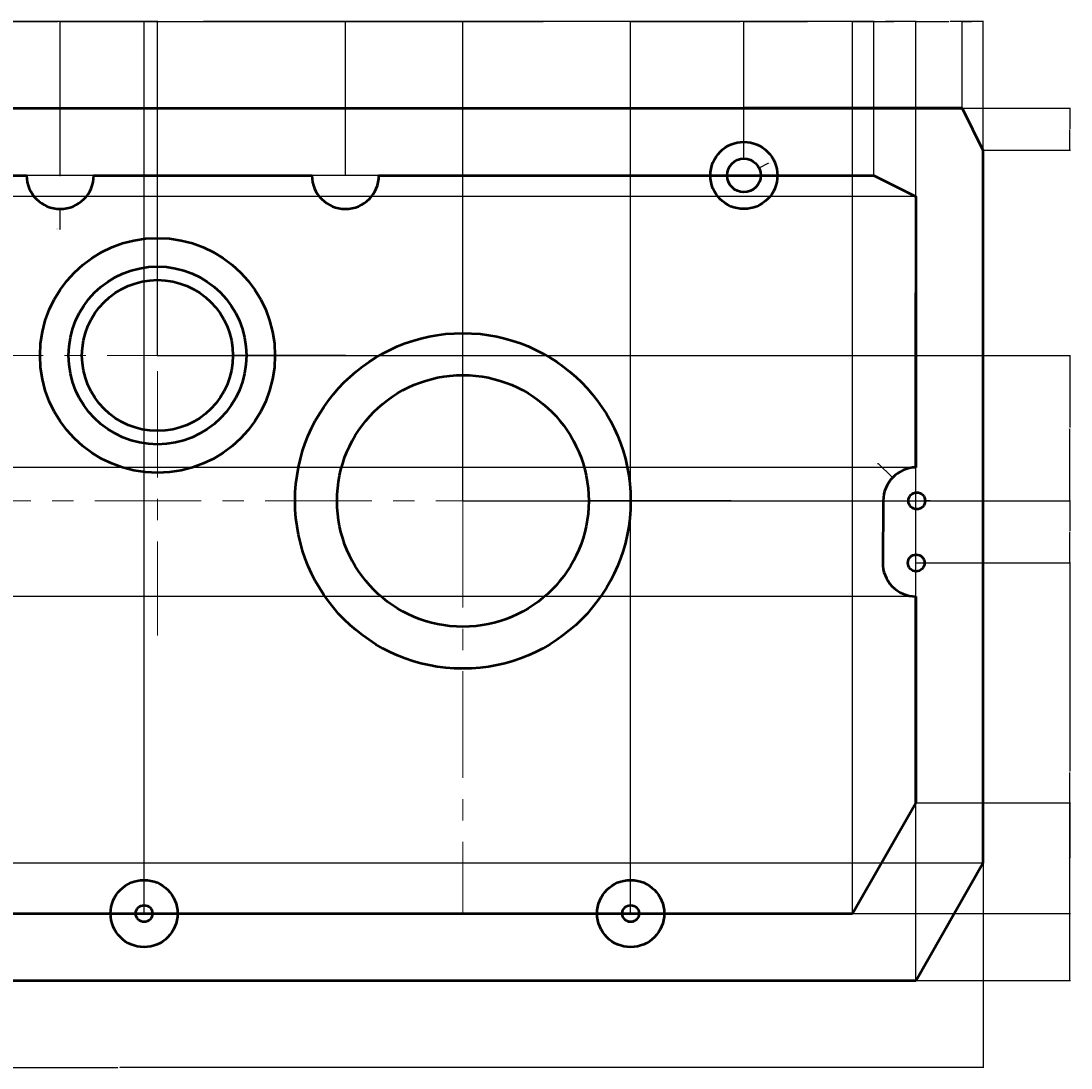
# Model space of a CAD drawing. Units: millimetres. Extents: x 2135 to 2702, y 2076 to 2388.
# Tile 2 of 2: x 2390 to 2702, y 2076 to 2388. Entities that reach past the tile are written whole.
import ezdxf

# ---------------------------------------------------------------- set-up
doc = ezdxf.new("R2010")
doc.units = ezdxf.units.MM
doc.linetypes.add('CENTER', pattern=[50.8, 31.75, -6.35, 6.35, -6.35])
for name, color, linetype, lineweight in [('M-CNTR', 4, 'CENTER', 18), ('M-DIMS', 2, 'Continuous', 18), ('M-OUTL', 7, 'Continuous', 50)]:
    doc.layers.add(name, color=color, linetype=linetype, lineweight=lineweight)
doc.styles.get("Standard").update_dxf_attribs({"font": 'arial.ttf'})
doc.dimstyles.get("Standard").update_dxf_attribs({"dimtxt": 0.18, "dimasz": 0.18, "dimexe": 0.18, "dimexo": 0.0625, "dimgap": 0.09, "dimtad": 0, "dimtih": 1, "dimtoh": 1, "dimdec": 4, "dimzin": 0, "dimdsep": 46, "dimtxsty": 'Standard', "dimcen": 0.09, "dimadec": 0, "dimazin": 0, "dimtfac": 1, "dimtdec": 4, "dimtofl": 0, "dimtmove": 0, "dimatfit": 3, "dimfxl": 1, "dimtolj": 1, "dimtzin": 0, "dimarcsym": 0})

# ---------------------------------------------------------------- blocks, each defined once
blk = doc.blocks.new('BOLT-HOLE-CBORE')
for radius in [10, 2.5]:
    blk.add_circle((10, 10), radius)
blk = doc.blocks.new('*D2')
at = {"layer": 'Defpoints', "color": 0, "transparency": 16777216}
for p in [(2676.22, 2136.75), (2161.22, 2101.69), (2676.22, 2075.84)]:
    blk.add_point(p, dxfattribs=at)
at = {"layer": 'M-DIMS', "color": 0, "lineweight": -2, "transparency": 16777216}
for p, q in [((2676.22, 2136.68), (2676.22, 2075.66)), ((2161.22, 2101.62), (2161.22, 2075.66)), ((2161.4, 2075.84), (2418.43, 2075.84)), ((2676.04, 2075.84), (2419.01, 2075.84))]:
    blk.add_line(p, q, dxfattribs=at)
at = {"layer": 'M-DIMS', "color": 0, "transparency": 16777216}
for points in [[(2161.4, 2075.87), (2161.4, 2075.81), (2161.22, 2075.84)], [(2676.04, 2075.87), (2676.04, 2075.81), (2676.22, 2075.84)]]:
    blk.add_solid(points, dxfattribs=at)
at = {"layer": 'M-DIMS', "color": 0, "transparency": 16777216, "insert": (2418.72, 2075.84), "char_height": 0.18, "attachment_point": 5}
blk.add_mtext('\\A1;515', dxfattribs=at)
blk = doc.blocks.new('*D6')
at = {"layer": 'Defpoints', "color": 0, "transparency": 16777216}
for p in [(2426.22, 2387.54), (2301.22, 2121.69), (2426.22, 2121.69)]:
    blk.add_point(p, dxfattribs=at)
at = {"layer": 'M-DIMS', "color": 0, "lineweight": -2, "transparency": 16777216}
for p, q in [((2301.22, 2121.75), (2301.22, 2387.72)), ((2301.4, 2387.54), (2363.44, 2387.54)), ((2426.04, 2387.54), (2364, 2387.54)), ((2426.22, 2121.75), (2426.22, 2387.72))]:
    blk.add_line(p, q, dxfattribs=at)
at = {"layer": 'M-DIMS', "color": 0, "transparency": 16777216}
for points in [[(2301.4, 2387.57), (2301.4, 2387.51), (2301.22, 2387.54)], [(2426.04, 2387.57), (2426.04, 2387.51), (2426.22, 2387.54)]]:
    blk.add_solid(points, dxfattribs=at)
at = {"layer": 'M-DIMS', "color": 0, "transparency": 16777216, "insert": (2363.72, 2387.54), "char_height": 0.18, "attachment_point": 5}
blk.add_mtext('\\A1;125', dxfattribs=at)
blk = doc.blocks.new('*D7')
at = {"layer": 'Defpoints', "color": 0, "transparency": 16777216}
for p in [(2571.22, 2387.54), (2426.22, 2121.69), (2571.22, 2121.69)]:
    blk.add_point(p, dxfattribs=at)
at = {"layer": 'M-DIMS', "color": 0, "lineweight": -2, "transparency": 16777216}
for p, q in [((2426.22, 2121.75), (2426.22, 2387.72)), ((2426.4, 2387.54), (2498.44, 2387.54)), ((2571.04, 2387.54), (2499, 2387.54)), ((2571.22, 2121.75), (2571.22, 2387.72))]:
    blk.add_line(p, q, dxfattribs=at)
at = {"layer": 'M-DIMS', "color": 0, "transparency": 16777216}
for points in [[(2426.4, 2387.57), (2426.4, 2387.51), (2426.22, 2387.54)], [(2571.04, 2387.57), (2571.04, 2387.51), (2571.22, 2387.54)]]:
    blk.add_solid(points, dxfattribs=at)
at = {"layer": 'M-DIMS', "color": 0, "transparency": 16777216, "insert": (2498.72, 2387.54), "char_height": 0.18, "attachment_point": 5}
blk.add_mtext('\\A1;145', dxfattribs=at)
blk = doc.blocks.new('*D8')
at = {"layer": 'Defpoints', "color": 0, "transparency": 16777216}
for p in [(2637.37, 2387.54), (2571.22, 2121.69), (2637.37, 2121.69)]:
    blk.add_point(p, dxfattribs=at)
at = {"layer": 'M-DIMS', "color": 0, "lineweight": -2, "transparency": 16777216}
for p, q in [((2571.22, 2121.75), (2571.22, 2387.72)), ((2571.4, 2387.54), (2603.9, 2387.54)), ((2637.19, 2387.54), (2604.69, 2387.54)), ((2637.37, 2121.75), (2637.37, 2387.72))]:
    blk.add_line(p, q, dxfattribs=at)
at = {"layer": 'M-DIMS', "color": 0, "transparency": 16777216}
for points in [[(2571.4, 2387.57), (2571.4, 2387.51), (2571.22, 2387.54)], [(2637.19, 2387.57), (2637.19, 2387.51), (2637.37, 2387.54)]]:
    blk.add_solid(points, dxfattribs=at)
at = {"layer": 'M-DIMS', "color": 0, "transparency": 16777216, "insert": (2604.29, 2387.54), "char_height": 0.18, "attachment_point": 5}
blk.add_mtext('\\A1;66.15', dxfattribs=at)
blk = doc.blocks.new('*D9')
at = {"layer": 'Defpoints', "color": 0, "transparency": 16777216}
for p in [(2656.22, 2387.54), (2656.22, 2154.73), (2637.37, 2121.69)]:
    blk.add_point(p, dxfattribs=at)
at = {"layer": 'M-DIMS', "color": 0, "lineweight": -2, "transparency": 16777216}
for p, q in [((2637.37, 2121.75), (2637.37, 2387.72)), ((2637.55, 2387.54), (2646.41, 2387.54)), ((2656.04, 2387.54), (2647.18, 2387.54)), ((2656.22, 2154.79), (2656.22, 2387.72))]:
    blk.add_line(p, q, dxfattribs=at)
at = {"layer": 'M-DIMS', "color": 0, "transparency": 16777216}
for points in [[(2637.55, 2387.57), (2637.55, 2387.51), (2637.37, 2387.54)], [(2656.04, 2387.57), (2656.04, 2387.51), (2656.22, 2387.54)]]:
    blk.add_solid(points, dxfattribs=at)
at = {"layer": 'M-DIMS', "color": 0, "transparency": 16777216, "insert": (2646.79, 2387.54), "char_height": 0.18, "attachment_point": 5}
blk.add_mtext('\\A1;18.85', dxfattribs=at)
blk = doc.blocks.new('*D10')
at = {"layer": 'Defpoints', "color": 0, "transparency": 16777216}
for p in [(2676.22, 2387.54), (2676.22, 2136.75), (2656.22, 2101.69)]:
    blk.add_point(p, dxfattribs=at)
at = {"layer": 'M-DIMS', "color": 0, "lineweight": -2, "transparency": 16777216}
for p, q in [((2656.22, 2101.75), (2656.22, 2387.72)), ((2656.4, 2387.54), (2666, 2387.54)), ((2676.04, 2387.54), (2666.44, 2387.54)), ((2676.22, 2136.81), (2676.22, 2387.72))]:
    blk.add_line(p, q, dxfattribs=at)
at = {"layer": 'M-DIMS', "color": 0, "transparency": 16777216}
for points in [[(2656.4, 2387.57), (2656.4, 2387.51), (2656.22, 2387.54)], [(2676.04, 2387.57), (2676.04, 2387.51), (2676.22, 2387.54)]]:
    blk.add_solid(points, dxfattribs=at)
at = {"layer": 'M-DIMS', "color": 0, "transparency": 16777216, "insert": (2666.22, 2387.54), "char_height": 0.18, "attachment_point": 5}
blk.add_mtext('\\A1;20', dxfattribs=at)
blk = doc.blocks.new('*D13')
at = {"layer": 'Defpoints', "color": 0, "transparency": 16777216}
for p in [(2401.22, 2387.54), (2371.22, 2341.69), (2401.22, 2341.69)]:
    blk.add_point(p, dxfattribs=at)
at = {"layer": 'M-DIMS', "color": 0, "lineweight": -2, "transparency": 16777216}
for p, q in [((2371.22, 2341.75), (2371.22, 2387.72)), ((2371.4, 2387.54), (2386, 2387.54)), ((2401.04, 2387.54), (2386.44, 2387.54)), ((2401.22, 2341.75), (2401.22, 2387.72))]:
    blk.add_line(p, q, dxfattribs=at)
at = {"layer": 'M-DIMS', "color": 0, "transparency": 16777216}
for points in [[(2371.4, 2387.57), (2371.4, 2387.51), (2371.22, 2387.54)], [(2401.04, 2387.57), (2401.04, 2387.51), (2401.22, 2387.54)]]:
    blk.add_solid(points, dxfattribs=at)
at = {"layer": 'M-DIMS', "color": 0, "transparency": 16777216, "insert": (2386.22, 2387.54), "char_height": 0.18, "attachment_point": 5}
blk.add_mtext('\\A1;30', dxfattribs=at)
blk = doc.blocks.new('*D14')
at = {"layer": 'Defpoints', "color": 0, "transparency": 16777216}
for p in [(2486.22, 2387.54), (2401.22, 2341.69), (2486.22, 2341.69)]:
    blk.add_point(p, dxfattribs=at)
at = {"layer": 'M-DIMS', "color": 0, "lineweight": -2, "transparency": 16777216}
for p, q in [((2401.22, 2341.75), (2401.22, 2387.72)), ((2401.4, 2387.54), (2443.5, 2387.54)), ((2486.04, 2387.54), (2443.94, 2387.54)), ((2486.22, 2341.75), (2486.22, 2387.72))]:
    blk.add_line(p, q, dxfattribs=at)
at = {"layer": 'M-DIMS', "color": 0, "transparency": 16777216}
for points in [[(2401.4, 2387.57), (2401.4, 2387.51), (2401.22, 2387.54)], [(2486.04, 2387.57), (2486.04, 2387.51), (2486.22, 2387.54)]]:
    blk.add_solid(points, dxfattribs=at)
at = {"layer": 'M-DIMS', "color": 0, "transparency": 16777216, "insert": (2443.72, 2387.54), "char_height": 0.18, "attachment_point": 5}
blk.add_mtext('\\A1;85', dxfattribs=at)
blk = doc.blocks.new('*D15')
at = {"layer": 'Defpoints', "color": 0, "transparency": 16777216}
for p in [(2604.97, 2387.54), (2604.97, 2346.69), (2486.22, 2341.69)]:
    blk.add_point(p, dxfattribs=at)
at = {"layer": 'M-DIMS', "color": 0, "lineweight": -2, "transparency": 16777216}
for p, q in [((2486.22, 2341.75), (2486.22, 2387.72)), ((2486.4, 2387.54), (2545.14, 2387.54)), ((2604.79, 2387.54), (2546.05, 2387.54)), ((2604.97, 2346.75), (2604.97, 2387.72))]:
    blk.add_line(p, q, dxfattribs=at)
at = {"layer": 'M-DIMS', "color": 0, "transparency": 16777216}
for points in [[(2486.4, 2387.57), (2486.4, 2387.51), (2486.22, 2387.54)], [(2604.79, 2387.57), (2604.79, 2387.51), (2604.97, 2387.54)]]:
    blk.add_solid(points, dxfattribs=at)
at = {"layer": 'M-DIMS', "color": 0, "transparency": 16777216, "insert": (2545.59, 2387.54), "char_height": 0.18, "attachment_point": 5}
blk.add_mtext('\\A1;118.75', dxfattribs=at)
blk = doc.blocks.new('*D16')
at = {"layer": 'Defpoints', "color": 0, "transparency": 16777216}
for p in [(2643.72, 2387.54), (2604.97, 2346.69), (2643.72, 2341.69)]:
    blk.add_point(p, dxfattribs=at)
at = {"layer": 'M-DIMS', "color": 0, "lineweight": -2, "transparency": 16777216}
for p, q in [((2604.97, 2346.75), (2604.97, 2387.72)), ((2605.15, 2387.54), (2623.95, 2387.54)), ((2643.54, 2387.54), (2624.74, 2387.54)), ((2643.72, 2341.75), (2643.72, 2387.72))]:
    blk.add_line(p, q, dxfattribs=at)
at = {"layer": 'M-DIMS', "color": 0, "transparency": 16777216}
for points in [[(2605.15, 2387.57), (2605.15, 2387.51), (2604.97, 2387.54)], [(2643.54, 2387.57), (2643.54, 2387.51), (2643.72, 2387.54)]]:
    blk.add_solid(points, dxfattribs=at)
at = {"layer": 'M-DIMS', "color": 0, "transparency": 16777216, "insert": (2624.34, 2387.54), "char_height": 0.18, "attachment_point": 5}
blk.add_mtext('\\A1;38.75', dxfattribs=at)
blk = doc.blocks.new('*D17')
at = {"layer": 'Defpoints', "color": 0, "transparency": 16777216}
for p in [(2656.22, 2387.54), (2643.72, 2341.69), (2656.22, 2335.44)]:
    blk.add_point(p, dxfattribs=at)
at = {"layer": 'M-DIMS', "color": 0, "lineweight": -2, "transparency": 16777216}
for p, q in [((2643.72, 2341.75), (2643.72, 2387.72)), ((2643.9, 2387.54), (2649.65, 2387.54)), ((2656.04, 2387.54), (2650.28, 2387.54)), ((2656.22, 2335.5), (2656.22, 2387.72))]:
    blk.add_line(p, q, dxfattribs=at)
at = {"layer": 'M-DIMS', "color": 0, "transparency": 16777216}
for points in [[(2643.9, 2387.57), (2643.9, 2387.51), (2643.72, 2387.54)], [(2656.04, 2387.57), (2656.04, 2387.51), (2656.22, 2387.54)]]:
    blk.add_solid(points, dxfattribs=at)
at = {"layer": 'M-DIMS', "color": 0, "transparency": 16777216, "insert": (2649.97, 2387.54), "char_height": 0.18, "attachment_point": 5}
blk.add_mtext('\\A1;12.5', dxfattribs=at)
blk = doc.blocks.new('*D18')
at = {"layer": 'Defpoints', "color": 0, "transparency": 16777216}
for p in [(2676.22, 2387.54), (2669.97, 2361.69), (2676.22, 2349.19)]:
    blk.add_point(p, dxfattribs=at)
at = {"layer": 'M-DIMS', "color": 0, "lineweight": -2, "transparency": 16777216}
for p, q in [((2669.97, 2361.75), (2669.97, 2387.72)), ((2670.15, 2387.54), (2672.77, 2387.54)), ((2676.04, 2387.54), (2673.42, 2387.54)), ((2676.22, 2349.25), (2676.22, 2387.72))]:
    blk.add_line(p, q, dxfattribs=at)
at = {"layer": 'M-DIMS', "color": 0, "transparency": 16777216}
for points in [[(2670.15, 2387.57), (2670.15, 2387.51), (2669.97, 2387.54)], [(2676.04, 2387.57), (2676.04, 2387.51), (2676.22, 2387.54)]]:
    blk.add_solid(points, dxfattribs=at)
at = {"layer": 'M-DIMS', "color": 0, "transparency": 16777216, "insert": (2673.09, 2387.54), "char_height": 0.18, "attachment_point": 5}
blk.add_mtext('\\A1;6.25', dxfattribs=at)
blk = doc.blocks.new('*D19')
at = {"layer": 'Defpoints', "color": 0, "transparency": 16777216}
for p in [(2430.22, 2387.54), (2371.22, 2306.69), (2430.22, 2288.03)]:
    blk.add_point(p, dxfattribs=at)
at = {"layer": 'M-DIMS', "color": 0, "lineweight": -2, "transparency": 16777216}
for p, q in [((2371.22, 2306.75), (2371.22, 2387.72)), ((2371.4, 2387.54), (2400.5, 2387.54)), ((2430.04, 2387.54), (2400.94, 2387.54)), ((2430.22, 2288.1), (2430.22, 2387.72))]:
    blk.add_line(p, q, dxfattribs=at)
at = {"layer": 'M-DIMS', "color": 0, "transparency": 16777216}
for points in [[(2371.4, 2387.57), (2371.4, 2387.51), (2371.22, 2387.54)], [(2430.04, 2387.57), (2430.04, 2387.51), (2430.22, 2387.54)]]:
    blk.add_solid(points, dxfattribs=at)
at = {"layer": 'M-DIMS', "color": 0, "transparency": 16777216, "insert": (2400.72, 2387.54), "char_height": 0.18, "attachment_point": 5}
blk.add_mtext('\\A1;59', dxfattribs=at)
blk = doc.blocks.new('*D20')
at = {"layer": 'Defpoints', "color": 0, "transparency": 16777216}
for p in [(2521.22, 2387.54), (2430.22, 2288.03), (2521.22, 2244.69)]:
    blk.add_point(p, dxfattribs=at)
at = {"layer": 'M-DIMS', "color": 0, "lineweight": -2, "transparency": 16777216}
for p, q in [((2430.22, 2288.1), (2430.22, 2387.72)), ((2430.4, 2387.54), (2475.52, 2387.54)), ((2521.04, 2387.54), (2475.92, 2387.54)), ((2521.22, 2244.75), (2521.22, 2387.72))]:
    blk.add_line(p, q, dxfattribs=at)
at = {"layer": 'M-DIMS', "color": 0, "transparency": 16777216}
for points in [[(2430.4, 2387.57), (2430.4, 2387.51), (2430.22, 2387.54)], [(2521.04, 2387.57), (2521.04, 2387.51), (2521.22, 2387.54)]]:
    blk.add_solid(points, dxfattribs=at)
at = {"layer": 'M-DIMS', "color": 0, "transparency": 16777216, "insert": (2475.72, 2387.54), "char_height": 0.18, "attachment_point": 5}
blk.add_mtext('\\A1;91', dxfattribs=at)
blk = doc.blocks.new('*D22')
at = {"layer": 'Defpoints', "color": 0, "transparency": 16777216}
for p in [(2637.37, 2121.69), (2135.37, 2101.69), (2656.22, 2101.69)]:
    blk.add_point(p, dxfattribs=at)
at = {"layer": 'M-DIMS', "color": 0, "lineweight": -2, "transparency": 16777216}
for p, q in [((2637.3, 2121.69), (2135.19, 2121.69)), ((2135.37, 2121.51), (2135.37, 2111.87)), ((2135.37, 2101.87), (2135.37, 2111.5)), ((2656.15, 2101.69), (2135.19, 2101.69))]:
    blk.add_line(p, q, dxfattribs=at)
at = {"layer": 'M-DIMS', "color": 0, "transparency": 16777216}
for points in [[(2135.34, 2121.51), (2135.4, 2121.51), (2135.37, 2121.69)], [(2135.34, 2101.87), (2135.4, 2101.87), (2135.37, 2101.69)]]:
    blk.add_solid(points, dxfattribs=at)
at = {"layer": 'M-DIMS', "color": 0, "transparency": 16777216, "insert": (2135.37, 2111.69), "char_height": 0.18, "attachment_point": 5}
blk.add_mtext('\\A1;20', dxfattribs=at)
blk = doc.blocks.new('*D27')
at = {"layer": 'Defpoints', "color": 0, "transparency": 16777216}
for p in [(2656.33, 2226.19), (2702.07, 2226.19), (2656.22, 2101.69)]:
    blk.add_point(p, dxfattribs=at)
at = {"layer": 'M-DIMS', "color": 0, "lineweight": -2, "transparency": 16777216}
for p, q in [((2656.39, 2226.19), (2702.25, 2226.19)), ((2702.07, 2226.01), (2702.07, 2164.12)), ((2702.07, 2101.87), (2702.07, 2163.75)), ((2656.28, 2101.69), (2702.25, 2101.69))]:
    blk.add_line(p, q, dxfattribs=at)
at = {"layer": 'M-DIMS', "color": 0, "transparency": 16777216}
for points in [[(2702.04, 2226.01), (2702.1, 2226.01), (2702.07, 2226.19)], [(2702.04, 2101.87), (2702.1, 2101.87), (2702.07, 2101.69)]]:
    blk.add_solid(points, dxfattribs=at)
at = {"layer": 'M-DIMS', "color": 0, "transparency": 16777216, "insert": (2702.07, 2163.94), "char_height": 0.18, "attachment_point": 5}
blk.add_mtext('\\A1;124.5', dxfattribs=at)
blk = doc.blocks.new('*D28')
at = {"layer": 'Defpoints', "color": 0, "transparency": 16777216}
for p in [(2521.22, 2244.69), (2702.07, 2244.69), (2656.33, 2226.19)]:
    blk.add_point(p, dxfattribs=at)
at = {"layer": 'M-DIMS', "color": 0, "lineweight": -2, "transparency": 16777216}
for p, q in [((2521.28, 2244.69), (2702.25, 2244.69)), ((2702.07, 2244.51), (2702.07, 2235.62)), ((2702.07, 2226.37), (2702.07, 2235.25)), ((2656.39, 2226.19), (2702.25, 2226.19))]:
    blk.add_line(p, q, dxfattribs=at)
at = {"layer": 'M-DIMS', "color": 0, "transparency": 16777216}
for points in [[(2702.04, 2244.51), (2702.1, 2244.51), (2702.07, 2244.69)], [(2702.04, 2226.37), (2702.1, 2226.37), (2702.07, 2226.19)]]:
    blk.add_solid(points, dxfattribs=at)
at = {"layer": 'M-DIMS', "color": 0, "transparency": 16777216, "insert": (2702.07, 2235.44), "char_height": 0.18, "attachment_point": 5}
blk.add_mtext('\\A1;18.5', dxfattribs=at)
blk = doc.blocks.new('*D29')
at = {"layer": 'Defpoints', "color": 0, "transparency": 16777216}
for p in [(2430.22, 2288.03), (2702.07, 2288.03), (2521.22, 2244.69)]:
    blk.add_point(p, dxfattribs=at)
at = {"layer": 'M-DIMS', "color": 0, "lineweight": -2, "transparency": 16777216}
for p, q in [((2430.28, 2288.03), (2702.25, 2288.03)), ((2702.07, 2287.85), (2702.07, 2266.54)), ((2702.07, 2244.87), (2702.07, 2266.18)), ((2521.28, 2244.69), (2702.25, 2244.69))]:
    blk.add_line(p, q, dxfattribs=at)
at = {"layer": 'M-DIMS', "color": 0, "transparency": 16777216}
for points in [[(2702.04, 2287.85), (2702.1, 2287.85), (2702.07, 2288.03)], [(2702.04, 2244.87), (2702.1, 2244.87), (2702.07, 2244.69)]]:
    blk.add_solid(points, dxfattribs=at)
at = {"layer": 'M-DIMS', "color": 0, "transparency": 16777216, "insert": (2702.07, 2266.36), "char_height": 0.18, "attachment_point": 5}
blk.add_mtext('\\A1;43.35', dxfattribs=at)
blk = doc.blocks.new('*D30')
at = {"layer": 'Defpoints', "color": 0, "transparency": 16777216}
for p in [(2135.37, 2254.68), (2656.22, 2254.68), (2656.22, 2216.19)]:
    blk.add_point(p, dxfattribs=at)
at = {"layer": 'M-DIMS', "color": 0, "lineweight": -2, "transparency": 16777216}
for p, q in [((2656.15, 2254.68), (2135.19, 2254.68)), ((2135.37, 2254.5), (2135.37, 2235.62)), ((2135.37, 2216.37), (2135.37, 2235.25)), ((2656.15, 2216.19), (2135.19, 2216.19))]:
    blk.add_line(p, q, dxfattribs=at)
at = {"layer": 'M-DIMS', "color": 0, "transparency": 16777216}
for points in [[(2135.34, 2254.5), (2135.4, 2254.5), (2135.37, 2254.68)], [(2135.34, 2216.37), (2135.4, 2216.37), (2135.37, 2216.19)]]:
    blk.add_solid(points, dxfattribs=at)
at = {"layer": 'M-DIMS', "color": 0, "transparency": 16777216, "insert": (2135.37, 2235.43), "char_height": 0.18, "attachment_point": 5}
blk.add_mtext('\\A1;38.495', dxfattribs=at)
blk = doc.blocks.new('*D31')
at = {"layer": 'Defpoints', "color": 0, "transparency": 16777216}
for p in [(2135.37, 2136.75), (2676.22, 2136.75), (2656.22, 2101.69)]:
    blk.add_point(p, dxfattribs=at)
at = {"layer": 'M-DIMS', "color": 0, "lineweight": -2, "transparency": 16777216}
for p, q in [((2676.15, 2136.75), (2135.19, 2136.75)), ((2135.37, 2136.57), (2135.37, 2119.4)), ((2135.37, 2101.87), (2135.37, 2119.03)), ((2656.15, 2101.69), (2135.19, 2101.69))]:
    blk.add_line(p, q, dxfattribs=at)
at = {"layer": 'M-DIMS', "color": 0, "transparency": 16777216}
for points in [[(2135.34, 2136.57), (2135.4, 2136.57), (2135.37, 2136.75)], [(2135.34, 2101.87), (2135.4, 2101.87), (2135.37, 2101.69)]]:
    blk.add_solid(points, dxfattribs=at)
at = {"layer": 'M-DIMS', "color": 0, "transparency": 16777216, "insert": (2135.37, 2119.22), "char_height": 0.18, "attachment_point": 5}
blk.add_mtext('\\A1;35.06', dxfattribs=at)
blk = doc.blocks.new('*D32')
at = {"layer": 'Defpoints', "color": 0, "transparency": 16777216}
for p in [(2656.22, 2154.73), (2702.07, 2154.73), (2637.37, 2121.69)]:
    blk.add_point(p, dxfattribs=at)
at = {"layer": 'M-DIMS', "color": 0, "lineweight": -2, "transparency": 16777216}
for p, q in [((2656.28, 2154.73), (2702.25, 2154.73)), ((2702.07, 2154.55), (2702.07, 2138.39)), ((2702.07, 2121.87), (2702.07, 2138.03)), ((2637.43, 2121.69), (2702.25, 2121.69))]:
    blk.add_line(p, q, dxfattribs=at)
at = {"layer": 'M-DIMS', "color": 0, "transparency": 16777216}
for points in [[(2702.04, 2154.55), (2702.1, 2154.55), (2702.07, 2154.73)], [(2702.04, 2121.87), (2702.1, 2121.87), (2702.07, 2121.69)]]:
    blk.add_solid(points, dxfattribs=at)
at = {"layer": 'M-DIMS', "color": 0, "transparency": 16777216, "insert": (2702.07, 2138.21), "char_height": 0.18, "attachment_point": 5}
blk.add_mtext('\\A1;33.045', dxfattribs=at)
blk = doc.blocks.new('*D33')
at = {"layer": 'Defpoints', "color": 0, "transparency": 16777216}
for p in [(2669.97, 2361.69), (2676.22, 2349.19), (2702.07, 2349.19)]:
    blk.add_point(p, dxfattribs=at)
at = {"layer": 'M-DIMS', "color": 0, "lineweight": -2, "transparency": 16777216}
for p, q in [((2670.03, 2361.69), (2702.25, 2361.69)), ((2702.07, 2361.51), (2702.07, 2355.62)), ((2702.07, 2349.37), (2702.07, 2355.25)), ((2676.28, 2349.19), (2702.25, 2349.19))]:
    blk.add_line(p, q, dxfattribs=at)
at = {"layer": 'M-DIMS', "color": 0, "transparency": 16777216}
for points in [[(2702.04, 2361.51), (2702.1, 2361.51), (2702.07, 2361.69)], [(2702.04, 2349.37), (2702.1, 2349.37), (2702.07, 2349.19)]]:
    blk.add_solid(points, dxfattribs=at)
at = {"layer": 'M-DIMS', "color": 0, "transparency": 16777216, "insert": (2702.07, 2355.44), "char_height": 0.18, "attachment_point": 5}
blk.add_mtext('\\A1;12.5', dxfattribs=at)
blk = doc.blocks.new('*D34')
at = {"layer": 'Defpoints', "color": 0, "transparency": 16777216}
for p in [(2643.72, 2341.69), (2135.37, 2335.44), (2656.22, 2335.44)]:
    blk.add_point(p, dxfattribs=at)
at = {"layer": 'M-DIMS', "color": 0, "lineweight": -2, "transparency": 16777216}
for p, q in [((2643.65, 2341.69), (2135.19, 2341.69)), ((2135.37, 2341.51), (2135.37, 2338.74)), ((2135.37, 2335.62), (2135.37, 2338.38)), ((2656.15, 2335.44), (2135.19, 2335.44))]:
    blk.add_line(p, q, dxfattribs=at)
at = {"layer": 'M-DIMS', "color": 0, "transparency": 16777216}
for points in [[(2135.34, 2341.51), (2135.4, 2341.51), (2135.37, 2341.69)], [(2135.34, 2335.62), (2135.4, 2335.62), (2135.37, 2335.44)]]:
    blk.add_solid(points, dxfattribs=at)
at = {"layer": 'M-DIMS', "color": 0, "transparency": 16777216, "insert": (2135.37, 2338.56), "char_height": 0.18, "attachment_point": 5}
blk.add_mtext('\\A1;6.25', dxfattribs=at)
blk = doc.blocks.new('*D35')
at = {"layer": 'Defpoints', "color": 0, "transparency": 16777216}
for p in [(2471.22, 2244.67), (2571.22, 2244.7)]:
    blk.add_point(p, dxfattribs=at)
at = {"layer": 'M-DIMS', "color": 0, "lineweight": -2, "transparency": 16777216}
for p, q in [((2521.13, 2244.69), (2521.31, 2244.69)), ((2521.22, 2244.6), (2521.22, 2244.78)), ((2601.22, 2244.71), (2571.4, 2244.7))]:
    blk.add_line(p, q, dxfattribs=at)
at = {"layer": 'M-DIMS', "color": 0, "transparency": 16777216}
blk.add_solid([(2571.4, 2244.73), (2571.4, 2244.67), (2571.22, 2244.7)], dxfattribs=at)
at = {"layer": 'M-DIMS', "color": 0, "transparency": 16777216, "insert": (2601.6, 2244.71), "char_height": 0.18, "attachment_point": 5}
blk.add_mtext('\\A1;∅100', dxfattribs=at)
blk = doc.blocks.new('*D36')
at = {"layer": 'Defpoints', "color": 0, "transparency": 16777216}
for p in [(2483.72, 2244.67), (2558.72, 2244.7)]:
    blk.add_point(p, dxfattribs=at)
at = {"layer": 'M-DIMS', "color": 0, "lineweight": -2, "transparency": 16777216}
for p, q in [((2521.13, 2244.69), (2521.31, 2244.69)), ((2521.22, 2244.6), (2521.22, 2244.78)), ((2581.22, 2244.71), (2558.9, 2244.7))]:
    blk.add_line(p, q, dxfattribs=at)
at = {"layer": 'M-DIMS', "color": 0, "transparency": 16777216}
blk.add_solid([(2558.9, 2244.73), (2558.9, 2244.67), (2558.72, 2244.7)], dxfattribs=at)
at = {"layer": 'M-DIMS', "color": 0, "transparency": 16777216, "insert": (2581.53, 2244.71), "char_height": 0.18, "attachment_point": 5}
blk.add_mtext('\\A1;∅75', dxfattribs=at)
blk = doc.blocks.new('*D37')
at = {"layer": 'Defpoints', "color": 0, "transparency": 16777216}
for p in [(2395.22, 2288.07), (2465.22, 2288)]:
    blk.add_point(p, dxfattribs=at)
at = {"layer": 'M-DIMS', "color": 0, "lineweight": -2, "transparency": 16777216}
for p, q in [((2430.13, 2288.03), (2430.31, 2288.03)), ((2430.22, 2287.94), (2430.22, 2288.12)), ((2486.22, 2287.98), (2465.4, 2288))]:
    blk.add_line(p, q, dxfattribs=at)
at = {"layer": 'M-DIMS', "color": 0, "transparency": 16777216}
blk.add_solid([(2465.4, 2288.03), (2465.4, 2287.97), (2465.22, 2288)], dxfattribs=at)
at = {"layer": 'M-DIMS', "color": 0, "transparency": 16777216, "insert": (2486.53, 2287.98), "char_height": 0.18, "attachment_point": 5}
blk.add_mtext('\\A1;∅70', dxfattribs=at)
blk = doc.blocks.new('*D38')
at = {"layer": 'Defpoints', "color": 0, "transparency": 16777216}
for p in [(2403.72, 2288.07), (2456.72, 2288)]:
    blk.add_point(p, dxfattribs=at)
at = {"layer": 'M-DIMS', "color": 0, "lineweight": -2, "transparency": 16777216}
for p, q in [((2430.13, 2288.03), (2430.31, 2288.03)), ((2430.22, 2287.94), (2430.22, 2288.12)), ((2472.62, 2287.98), (2456.9, 2288))]:
    blk.add_line(p, q, dxfattribs=at)
at = {"layer": 'M-DIMS', "color": 0, "transparency": 16777216}
blk.add_solid([(2456.9, 2288.03), (2456.9, 2287.97), (2456.72, 2288)], dxfattribs=at)
at = {"layer": 'M-DIMS', "color": 0, "transparency": 16777216, "insert": (2472.93, 2287.98), "char_height": 0.18, "attachment_point": 5}
blk.add_mtext('\\A1;∅53', dxfattribs=at)
blk = doc.blocks.new('*D39')
at = {"layer": 'Defpoints', "color": 0, "transparency": 16777216}
for p in [(2407.72, 2288.07), (2452.72, 2288)]:
    blk.add_point(p, dxfattribs=at)
at = {"layer": 'M-DIMS', "color": 0, "lineweight": -2, "transparency": 16777216}
for p, q in [((2430.13, 2288.03), (2430.31, 2288.03)), ((2430.22, 2287.94), (2430.22, 2288.12)), ((2466.22, 2287.98), (2452.9, 2288))]:
    blk.add_line(p, q, dxfattribs=at)
at = {"layer": 'M-DIMS', "color": 0, "transparency": 16777216}
blk.add_solid([(2452.9, 2288.03), (2452.9, 2287.97), (2452.72, 2288)], dxfattribs=at)
at = {"layer": 'M-DIMS', "color": 0, "transparency": 16777216, "insert": (2466.53, 2287.98), "char_height": 0.18, "attachment_point": 5}
blk.add_mtext('\\A1;∅45', dxfattribs=at)
blk = doc.blocks.new('*D40')
at = {"layer": 'Defpoints', "color": 0, "transparency": 16777216}
for p in [(2416.22, 2121.67), (2436.22, 2121.7)]:
    blk.add_point(p, dxfattribs=at)
at = {"layer": 'M-DIMS', "color": 0, "lineweight": -2, "transparency": 16777216}
for p, q in [((2426.13, 2121.69), (2426.31, 2121.69)), ((2426.22, 2121.6), (2426.22, 2121.78)), ((2442.22, 2121.71), (2436.4, 2121.7))]:
    blk.add_line(p, q, dxfattribs=at)
at = {"layer": 'M-DIMS', "color": 0, "transparency": 16777216}
blk.add_solid([(2436.4, 2121.73), (2436.4, 2121.67), (2436.22, 2121.7)], dxfattribs=at)
at = {"layer": 'M-DIMS', "color": 0, "transparency": 16777216, "insert": (2442.73, 2121.71), "char_height": 0.18, "attachment_point": 5}
blk.add_mtext('\\A1;4X ∅20', dxfattribs=at)
blk = doc.blocks.new('*D42')
at = {"layer": 'Defpoints', "color": 0, "transparency": 16777216}
for p in [(2609.44, 2343.92), (2600.49, 2339.45)]:
    blk.add_point(p, dxfattribs=at)
at = {"layer": 'M-DIMS', "color": 0, "lineweight": -2, "transparency": 16777216}
for p, q in [((2612.12, 2345.26), (2609.6, 2344)), ((2612.3, 2345.26), (2612.12, 2345.26)), ((2604.88, 2341.69), (2605.06, 2341.69)), ((2604.97, 2341.6), (2604.97, 2341.78))]:
    blk.add_line(p, q, dxfattribs=at)
at = {"layer": 'M-DIMS', "color": 0, "transparency": 16777216}
blk.add_solid([(2609.59, 2344.03), (2609.61, 2343.97), (2609.44, 2343.92)], dxfattribs=at)
at = {"layer": 'M-DIMS', "color": 0, "transparency": 16777216, "insert": (2612.62, 2345.26), "char_height": 0.18, "attachment_point": 5}
blk.add_mtext('\\A1;∅10', dxfattribs=at)
blk = doc.blocks.new('*D45')
at = {"layer": 'Defpoints', "color": 0, "transparency": 16777216}
for p in [(2653.98, 2244.67), (2658.98, 2244.7)]:
    blk.add_point(p, dxfattribs=at)
at = {"layer": 'M-DIMS', "color": 0, "lineweight": -2, "transparency": 16777216}
for p, q in [((2656.39, 2244.69), (2656.57, 2244.69)), ((2656.48, 2244.6), (2656.48, 2244.78)), ((2660.48, 2244.71), (2659.16, 2244.7))]:
    blk.add_line(p, q, dxfattribs=at)
at = {"layer": 'M-DIMS', "color": 0, "transparency": 16777216}
blk.add_solid([(2659.16, 2244.73), (2659.16, 2244.67), (2658.98, 2244.7)], dxfattribs=at)
at = {"layer": 'M-DIMS', "color": 0, "transparency": 16777216, "insert": (2660.91, 2244.71), "char_height": 0.18, "attachment_point": 5}
blk.add_mtext('\\A1;2X ∅5', dxfattribs=at)
blk = doc.blocks.new('*D46')
at = {"layer": 'Defpoints', "color": 0, "transparency": 16777216}
for p in [(2401.22, 2341.69), (2401.19, 2331.69)]:
    blk.add_point(p, dxfattribs=at)
at = {"layer": 'M-DIMS', "color": 0, "lineweight": -2, "transparency": 16777216}
for p, q in [((2401.13, 2341.69), (2401.31, 2341.69)), ((2401.22, 2341.6), (2401.22, 2341.78)), ((2401.18, 2325.69), (2401.19, 2331.51)), ((2401, 2325.69), (2401.18, 2325.69))]:
    blk.add_line(p, q, dxfattribs=at)
at = {"layer": 'M-DIMS', "color": 0, "transparency": 16777216}
blk.add_solid([(2401.16, 2331.51), (2401.22, 2331.51), (2401.19, 2331.69)], dxfattribs=at)
at = {"layer": 'M-DIMS', "color": 0, "transparency": 16777216, "insert": (2400.5, 2325.69), "char_height": 0.18, "attachment_point": 5}
blk.add_mtext('\\A1;3X R10', dxfattribs=at)
blk = doc.blocks.new('*D47')
at = {"layer": 'Defpoints', "color": 0, "transparency": 16777216}
for p in [(2649.28, 2251.63), (2656.48, 2244.69)]:
    blk.add_point(p, dxfattribs=at)
at = {"layer": 'M-DIMS', "color": 0, "lineweight": -2, "transparency": 16777216}
for p, q in [((2644.78, 2255.79), (2644.96, 2255.79)), ((2644.96, 2255.79), (2649.15, 2251.75)), ((2656.39, 2244.69), (2656.57, 2244.69)), ((2656.48, 2244.6), (2656.48, 2244.78))]:
    blk.add_line(p, q, dxfattribs=at)
at = {"layer": 'M-DIMS', "color": 0, "transparency": 16777216}
blk.add_solid([(2649.17, 2251.77), (2649.13, 2251.73), (2649.28, 2251.63)], dxfattribs=at)
at = {"layer": 'M-DIMS', "color": 0, "transparency": 16777216, "insert": (2644.28, 2255.79), "char_height": 0.18, "attachment_point": 5}
blk.add_mtext('\\A1;2X R10', dxfattribs=at)

msp = doc.modelspace()

# ---------------------------------------------------------------- linework, layer by layer
at = {"layer": 'M-CNTR'}
for p, q in [((2430.2172, 2334.1854), (2430.2172, 2204.5212)), ((2161.2172, 2288.0325), (2416.86, 2288.0325)), ((2416.86, 2288.0325), (2456.1851, 2288.0325)), ((2646.4762, 2244.6854), (2292.5799, 2244.6854))]:
    msp.add_line(p, q, dxfattribs=at)
msp.add_lwpolyline([(2521.2172, 2244.6854), (2521.2172, 2121.6854)], dxfattribs=at)
at = {"layer": 'M-OUTL'}
for p, q in [((2669.9672, 2361.6854), (2604.9672, 2361.6854)), ((2676.2172, 2341.6854), (2676.2172, 2244.6854)), ((2646.4762, 2244.6854), (2646.3257, 2226.186)), ((2637.3663, 2121.6854), (2656.2172, 2154.7307)), ((2656.2172, 2101.6854), (2676.2172, 2136.745))]:
    msp.add_line(p, q, dxfattribs=at)
for points in [[(2656.2172, 2101.6854), (2161.2172, 2101.6854), (2161.2172, 2121.6854), (2161.2172, 2324.3525), (2161.2172, 2326.6854), (2181.2172, 2326.6854), (2351.2172, 2326.6854), (2351.2172, 2341.6854), (2351.2172, 2361.6854), (2371.2172, 2361.6854), (2669.9672, 2361.6854), (2676.2172, 2349.1854), (2676.2172, 2341.6854), (2676.2172, 2136.745)], [(2656.2172, 2254.6821), (2656.2172, 2306.6854)], [(2656.2172, 2154.7307), (2656.2172, 2216.1866)], [(2656.2172, 2216.1866), (2656.2172, 2154.7307)]]:
    msp.add_lwpolyline(points, dxfattribs=at)
for points in [[(2371.2172, 2306.6854), (2371.2172, 2341.6854), (2391.2172, 2341.6854, 1), (2411.2172, 2341.6854), (2476.2172, 2341.6854, 1), (2496.2172, 2341.6854), (2643.7172, 2341.6854), (2656.2172, 2335.4354), (2656.2172, 2254.6821)], [(2181.2172, 2226.6854), (2181.2172, 2131.6854, -0.41421356), (2191.2172, 2121.6854), (2637.3663, 2121.6854)]]:
    msp.add_lwpolyline(points, format="xyb", dxfattribs=at)
for centre, radius in [((2604.9672, 2341.6854), 10), ((2604.9672, 2341.6854), 5), ((2430.2172, 2288.0325), 35), ((2430.2172, 2288.0325), 26.5), ((2430.2172, 2288.0325), 22.5), ((2521.2172, 2244.6854), 50), ((2521.2172, 2244.6854), 37.5), ((2656.4762, 2244.6854), 2.5), ((2656.3257, 2226.186), 2.5)]:
    msp.add_circle(centre, radius, dxfattribs=at)
for centre, start, end in [((2656.4762, 2244.6854), 91.483946, 180), ((2656.3257, 2226.186), 179.067727, 269.37855)]:
    msp.add_arc(centre, 10, start, end, dxfattribs=at)

# ---------------------------------------------------------------- block references
for p in [(2416.217, 2111.685), (2561.217, 2111.685)]:
    msp.add_blockref('BOLT-HOLE-CBORE', p, dxfattribs=at)

# ---------------------------------------------------------------- dimensions: what is measured, and where the dimension line sits
at = {"layer": 'M-DIMS'}
for base, p1, p2, override, picture, middle in [((2426.2172, 2387.5354), (2301.2172, 2121.6854), (2426.2172, 2121.6854), {"dimdec": 0, "dimlfac": 1, "dimrnd": 0, "dimzin": 0, "dimdsep": 46, "dimlunit": 2}, '*D6', (2363.7172, 2387.5354)), ((2401.2172, 2387.5354), (2371.2172, 2341.6854), (2401.2172, 2341.6854), {"dimdec": 0, "dimlfac": 1, "dimrnd": 0, "dimzin": 0, "dimdsep": 46, "dimlunit": 2}, '*D13', (2386.2172, 2387.5354)), ((2430.2172, 2387.5354), (2371.2172, 2306.6854), (2430.2172, 2288.0325), {"dimdec": 0, "dimlfac": 1, "dimrnd": 0, "dimzin": 0, "dimdsep": 46, "dimlunit": 2}, '*D19', (2400.7172, 2387.5354)), ((2486.2172, 2387.5354), (2401.2172, 2341.6854), (2486.2172, 2341.6854), {"dimdec": 0, "dimlfac": 1, "dimrnd": 0, "dimzin": 0, "dimdsep": 46, "dimlunit": 2}, '*D14', (2443.7172, 2387.5354)), ((2571.2172, 2387.5354), (2426.2172, 2121.6854), (2571.2172, 2121.6854), {"dimdec": 0, "dimlfac": 1, "dimrnd": 0, "dimzin": 0, "dimdsep": 46, "dimlunit": 2}, '*D7', (2498.7172, 2387.5354)), ((2521.2172, 2387.5354), (2430.2172, 2288.0325), (2521.2172, 2244.6854), {"dimdec": 0, "dimlfac": 1, "dimrnd": 0, "dimzin": 0, "dimdsep": 46, "dimlunit": 2}, '*D20', (2475.7172, 2387.5354)), ((2604.9672, 2387.5354), (2486.2172, 2341.6854), (2604.9672, 2346.6854), {"dimdec": 2, "dimlfac": 1, "dimrnd": 0, "dimzin": 0, "dimdsep": 46, "dimlunit": 2}, '*D15', (2545.5922, 2387.5354)), ((2637.3663, 2387.5354), (2571.2172, 2121.6854), (2637.3663, 2121.6854), {"dimdec": 2, "dimlfac": 1, "dimrnd": 0, "dimzin": 0, "dimdsep": 46, "dimlunit": 2}, '*D8', (2604.2917, 2387.5354)), ((2643.7172, 2387.5354), (2604.9672, 2346.6854), (2643.7172, 2341.6854), {"dimdec": 2, "dimlfac": 1, "dimrnd": 0, "dimzin": 0, "dimdsep": 46, "dimlunit": 2}, '*D16', (2624.3422, 2387.5354)), ((2656.2172, 2387.5354), (2637.3663, 2121.6854), (2656.2172, 2154.7307), {"dimdec": 2, "dimlfac": 1, "dimrnd": 0, "dimzin": 0, "dimdsep": 46, "dimlunit": 2}, '*D9', (2646.7917, 2387.5354)), ((2656.2172, 2387.5354), (2643.7172, 2341.6854), (2656.2172, 2335.4354), {"dimdec": 1, "dimlfac": 1, "dimrnd": 0, "dimzin": 0, "dimdsep": 46, "dimlunit": 2}, '*D17', (2649.9672, 2387.5354)), ((2676.2172, 2387.5354), (2656.2172, 2101.6854), (2676.2172, 2136.745), {"dimdec": 0, "dimlfac": 1, "dimrnd": 0, "dimzin": 0, "dimdsep": 46, "dimlunit": 2}, '*D10', (2666.2172, 2387.5354)), ((2676.2172, 2387.5354), (2669.9672, 2361.6854), (2676.2172, 2349.1854), {"dimdec": 2, "dimlfac": 1, "dimrnd": 0, "dimzin": 0, "dimdsep": 46, "dimlunit": 2}, '*D18', (2673.0922, 2387.5354)), ((2676.2172, 2075.8354), (2161.2172, 2101.6854), (2676.2172, 2136.745), {"dimdec": 0, "dimlfac": 1, "dimrnd": 0, "dimzin": 0, "dimdsep": 46, "dimlunit": 2}, '*D2', (2418.7172, 2075.8354))]:
    dim = msp.add_linear_dim(base=base, p1=p1, p2=p2, dimstyle='Standard', override=override, dxfattribs=at)
    dim.commit()
    dim.dimension.update_dxf_attribs({"geometry": picture, "text_midpoint": middle})
for base, p1, p2, override, picture, middle in [((2702.0672, 2349.1854), (2669.9672, 2361.6854), (2676.2172, 2349.1854), {"dimdec": 1, "dimlfac": 1, "dimrnd": 0, "dimzin": 0, "dimdsep": 46, "dimlunit": 2}, '*D33', (2702.0672, 2355.4354)), ((2135.3672, 2335.4354), (2643.7172, 2341.6854), (2656.2172, 2335.4354), {"dimdec": 2, "dimlfac": 1, "dimrnd": 0, "dimzin": 0, "dimdsep": 46, "dimlunit": 2}, '*D34', (2135.3672, 2338.5604)), ((2702.0672, 2288.0325), (2521.2172, 2244.6854), (2430.2172, 2288.0325), {"dimdec": 2, "dimlfac": 1, "dimrnd": 0, "dimzin": 0, "dimdsep": 46, "dimlunit": 2}, '*D29', (2702.0672, 2266.359)), ((2135.3672, 2254.68207), (2656.2172, 2216.18662), (2656.2172, 2254.68207), {"dimdec": 3, "dimlfac": 1, "dimrnd": 0, "dimzin": 0, "dimdsep": 46, "dimlunit": 2}, '*D30', (2135.3672, 2235.43434)), ((2702.0672, 2244.6854), (2656.3257, 2226.186), (2521.2172, 2244.6854), {"dimdec": 1, "dimlfac": 1, "dimrnd": 0, "dimzin": 0, "dimdsep": 46, "dimlunit": 2}, '*D28', (2702.0672, 2235.4357)), ((2702.0672, 2226.186), (2656.2172, 2101.6854), (2656.3257, 2226.186), {"dimdec": 1, "dimlfac": 1, "dimrnd": 0, "dimzin": 0, "dimdsep": 46, "dimlunit": 2}, '*D27', (2702.0672, 2163.9357)), ((2702.0672, 2154.7307), (2637.3663, 2121.6854), (2656.2172, 2154.7307), {"dimdec": 3, "dimlfac": 1, "dimrnd": 0, "dimzin": 0, "dimdsep": 46, "dimlunit": 2}, '*D32', (2702.0672, 2138.2081)), ((2135.3672, 2136.745), (2656.2172, 2101.6854), (2676.2172, 2136.745), {"dimdec": 2, "dimlfac": 1, "dimrnd": 0, "dimzin": 0, "dimdsep": 46, "dimlunit": 2}, '*D31', (2135.3672, 2119.2152)), ((2135.3672, 2101.6854), (2637.3663, 2121.6854), (2656.2172, 2101.6854), {"dimdec": 0, "dimlfac": 1, "dimrnd": 0, "dimzin": 0, "dimdsep": 46, "dimlunit": 2}, '*D22', (2135.3672, 2111.6854))]:
    dim = msp.add_linear_dim(base=base, p1=p1, p2=p2, angle=90, dimstyle='Standard', override=override, dxfattribs=at)
    dim.commit()
    dim.dimension.update_dxf_attribs({"geometry": picture, "text_midpoint": middle})
for p1, p2, picture, middle in [((2600.4944, 2339.4506), (2609.44, 2343.9202), '*D42', (2612.6202, 2345.2611)), ((2395.2172, 2288.0651), (2465.2172, 2288), '*D37', (2486.2172, 2287.9805)), ((2403.7172, 2288.0651), (2456.7172, 2288), '*D38', (2472.6172, 2287.9805)), ((2407.7172, 2288.0651), (2452.7172, 2288), '*D39', (2466.2172, 2287.9804)), ((2471.2172, 2244.6708), (2571.2172, 2244.7), '*D35', (2601.2172, 2244.7088)), ((2483.7172, 2244.6708), (2558.7172, 2244.7), '*D36', (2581.2172, 2244.7088))]:
    dim = msp.add_diameter_dim_2p(p1=p1, p2=p2, dimstyle='Standard', override={"dimdec": 0, "dimlfac": 1, "dimrnd": 0, "dimzin": 0, "dimdsep": 46, "dimlunit": 2}, dxfattribs=at)
    dim.commit()
    dim.dimension.update_dxf_attribs({"geometry": picture, "text_midpoint": middle, "dimtype": 163})
for center, mpoint, text, picture, middle in [((2401.2172, 2341.6854), (2401.1942, 2331.6854), '3X <>', '*D46', (2400.5024, 2325.6855)), ((2656.4762, 2244.6854), (2649.2786, 2251.6277), '2X <>', '*D47', (2644.2804, 2255.7931))]:
    dim = msp.add_radius_dim(center=center, mpoint=mpoint, text=text, dimstyle='Standard', override={"dimdec": 0, "dimlfac": 1, "dimrnd": 0, "dimzin": 0, "dimdsep": 46, "dimlunit": 2}, dxfattribs=at)
    dim.commit()
    dim.dimension.update_dxf_attribs({"geometry": picture, "text_midpoint": middle, "dimtype": 164})
for p1, p2, text, picture, middle in [((2653.9762, 2244.671), (2658.9761, 2244.6999), '2X <>', '*D45', (2660.4761, 2244.7085)), ((2416.2172, 2121.6708), (2436.2172, 2121.7), '4X <>', '*D40', (2442.2172, 2121.7088))]:
    dim = msp.add_diameter_dim_2p(p1=p1, p2=p2, text=text, dimstyle='Standard', override={"dimdec": 0, "dimlfac": 1, "dimrnd": 0, "dimzin": 0, "dimdsep": 46, "dimlunit": 2}, dxfattribs=at)
    dim.commit()
    dim.dimension.update_dxf_attribs({"geometry": picture, "text_midpoint": middle, "dimtype": 163})

doc.saveas('drawing.dxf')
